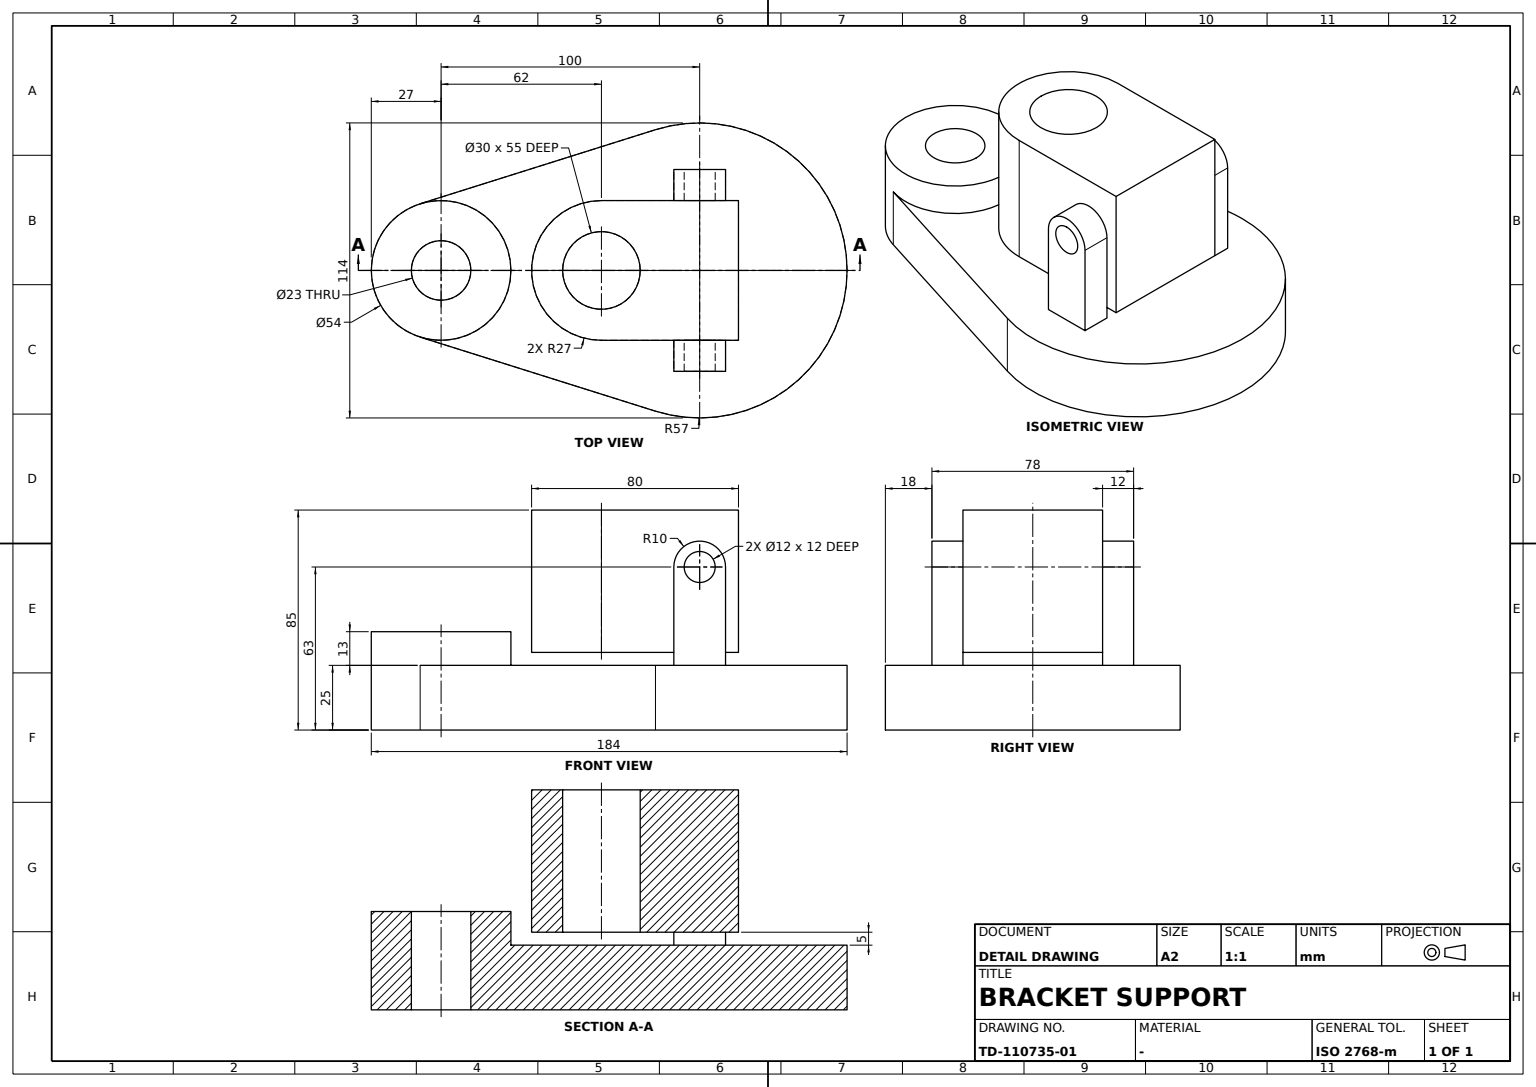
CATIA V5 part; units mm, degrees
sketch "Sketch1" plane through (0, 0, 0) normal (0, 0, 1) x (1, 0, 0)
  arc A0 (-8.1, 25.7564) -> (-8.1, -25.7564) centre (0, 0) ccw
  arc A1 (82.9, -54.3745) -> (82.9, 54.3745) centre (100, 0) ccw
  point P0 (100, 0)
  line L0 (-8.1, 25.7564) -> (82.9, 54.3745)
  line L1 (-8.1, -25.7564) -> (82.9, -54.3745)
  dimension "radius A0" = 27
  dimension "radius A1" = 57
  dimension "distance P0 y axis" = 100
  constraint coincidence P0 x-axis
  constraint tangency L0 A0
  constraint tangency L0 A1
  constraint tangency L1 A0
  constraint tangency L1 A1
extrude "Pad1" add sketch "Sketch1" along normal blind 25
sketch "Sketch2" plane through (0, 0, 25) normal (0, 0, 1) x (1, 0, 0)
  circle A0 centre (0, 0) radius 27
  arc A1 (-8.1, 25.7564) -> (-8.1, -25.7564) centre (0, 0) ccw construction
  arc A2 (-8.1, 25.7564) -> (-8.1, -25.7564) centre (0, 0) ccw construction
  circle A3 centre (0, 0) radius 11.5
  dimension "radius A3" = 11.5
  constraint concentricity A0 A1
  constraint concentricity A3 A0
  constraint coincidence A0 A2
extrude "Pad2" add sketch "Sketch2" along normal blind 13
extrude "MultiPocket1 domain 1" cut sketch "Sketch2" against normal blind 38 contours A3
sketch "Sketch3" plane through (0, 0, 25) normal (0, 0, 1) x (1, 0, 0)
  point P0 (100, 33)
  line L0 (110, 39) -> (110, 27)
  line L1 (110, 27) -> (90, 27)
  line L2 (90, 27) -> (90, 39)
  line L3 (90, 39) -> (110, 39)
  point P1 (110, 39)
  point P2 (110, 27)
  point P3 (90, 27)
  point P4 (90, 39)
  point P5 (100, -33)
  point P6 (110, -39)
  point P7 (110, -27)
  point P8 (90, -27)
  point P9 (90, -39)
  line L4 (110, -39) -> (110, -27)
  line L5 (110, -27) -> (90, -27)
  line L6 (90, -27) -> (90, -39)
  line L7 (90, -39) -> (110, -39)
  dimension "distance y axis P0" = 100
  dimension "distance L1 L3" = 12
  dimension "length L3" = 20
  dimension "distance P0 x axis" = 33
  constraint vertical L0 y-axis
  constraint vertical L2 y-axis
  constraint horizontal L1 x-axis
  constraint horizontal L3 x-axis
  constraint equidistance L0 L2 P0
  constraint equidistance L1 L3 P0
  constraint symmetry P0 P5 x-axis
  constraint symmetry P1 P6 x-axis
  constraint symmetry P2 P7 x-axis
  constraint symmetry P3 P8 x-axis
  constraint symmetry P4 P9 x-axis
  constraint symmetry L0 L4 x-axis
  constraint symmetry L1 L5 x-axis
  constraint symmetry L2 L6 x-axis
  constraint symmetry L3 L7 x-axis
extrude "Pad3" add sketch "Sketch3" along normal blind 48
fillet "Fillet1" radius 10 4 edges at (90, -33, 73) (110, -33, 73) (90, 33, 73) (110, 33, 73)
sketch "Sketch4" plane through (0, 39, 0) normal (0, 1, 0) x (-1, 0, 0)
  circle A0 centre (-100, 63) radius 6
  arc A1 (-100, 73) -> (-110, 63) centre (-100, 63) ccw construction
  dimension "radius A0" = 6
  constraint concentricity A0 A1
extrude "Pocket1" cut sketch "Sketch4" against normal through all
sketch "Sketch5" plane through (0, 0, 0) normal (0, 1, 0) x (-1, 0, 0)
  point P0 (-75, 57.5)
  line L0 (-35, 85) -> (-35, 30)
  line L1 (-35, 30) -> (-115, 30)
  line L2 (-115, 30) -> (-115, 85)
  line L3 (-115, 85) -> (-35, 85)
  line L4 (-157, 25) -> (-82.9, 25) construction
  line L5 (-157, 0) -> (-82.9, 0) construction
  dimension "distance L4 L1" = 5
  dimension "distance L5 L3" = 85
  dimension "length L3" = 80
  dimension "D4" = 35
  constraint vertical L0 y-axis
  constraint vertical L2 y-axis
  constraint horizontal L1 x-axis
  constraint horizontal L3 x-axis
  constraint equidistance L0 L2 P0
  constraint equidistance L1 L3 P0
extrude "Pad4" add sketch "Sketch5" along normal mid plane 54
fillet "Fillet2" radius 27 2 edges at (35, 27, 57.5) (35, -27, 57.5)
sketch "Sketch6" plane through (58.2107, 6.6311, 85) normal (0, 0, 1) x (1, 0, 0)
  point P0 (3.7893, -6.6311)
  arc A0 (3.7893, 20.3689) -> (-23.2107, -6.6311) centre (3.7893, -6.6311) ccw construction
  constraint concentricity P0 A0
hole "Hole1" at (62, 0, 85) direction (0, 0, -1) diameter 30 depth 57
